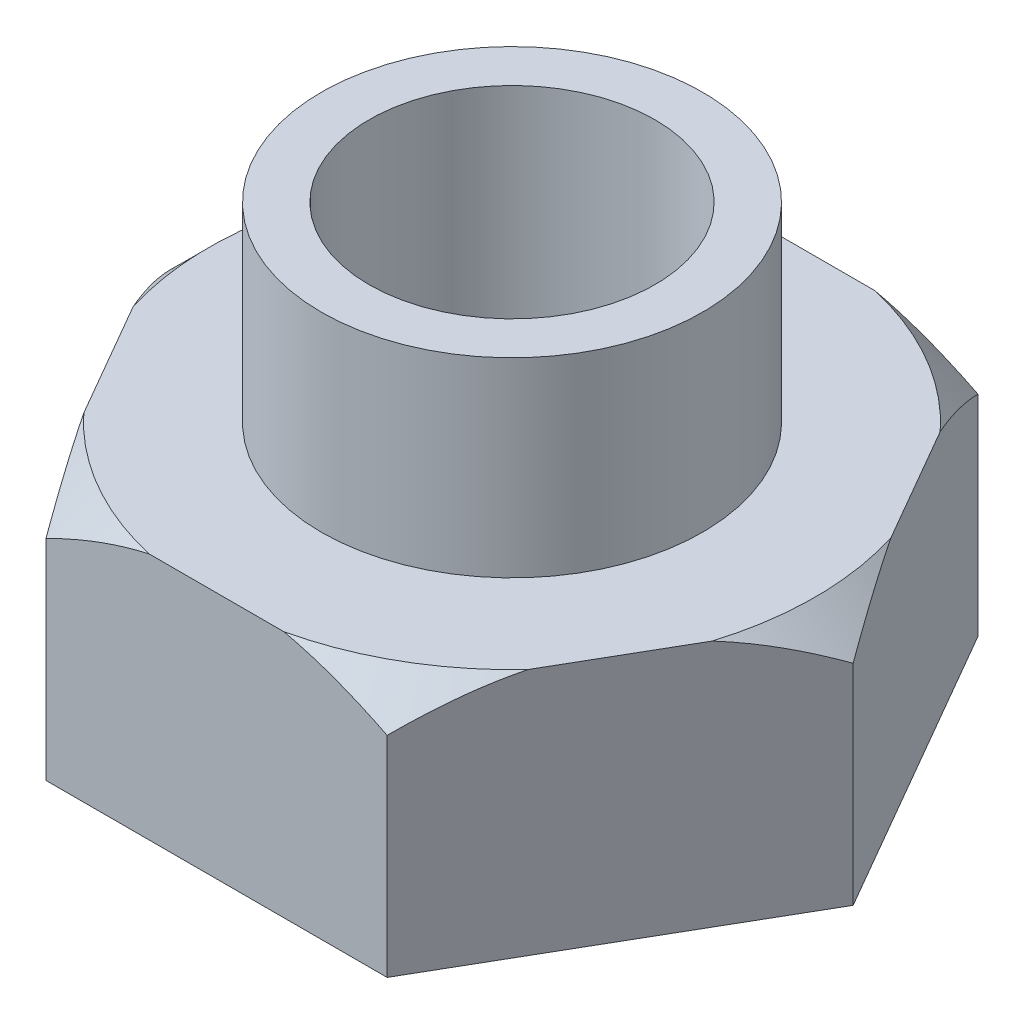
ISO-10303-21;
HEADER;
FILE_DESCRIPTION(('STEP AP214'),'2;1');
FILE_NAME('part.step','',(''),(''),'','','');
FILE_SCHEMA(('AUTOMOTIVE_DESIGN { 1 0 10303 214 1 1 1 1 }'));
ENDSEC;
DATA;
#1=APPLICATION_CONTEXT('core data for automotive mechanical design processes');
#2=APPLICATION_PROTOCOL_DEFINITION('international standard','automotive_design',2000,#1);
#3=PRODUCT_CONTEXT('',#1,'mechanical');
#4=PRODUCT('Part','Part','',(#3));
#5=PRODUCT_RELATED_PRODUCT_CATEGORY('part','',(#4));
#6=PRODUCT_DEFINITION_FORMATION('','',#4);
#7=PRODUCT_DEFINITION_CONTEXT('part definition',#1,'design');
#8=PRODUCT_DEFINITION('design','',#6,#7);
#9=PRODUCT_DEFINITION_SHAPE('','',#8);
#10=(LENGTH_UNIT() NAMED_UNIT(*) SI_UNIT(.MILLI.,.METRE.));
#11=(NAMED_UNIT(*) PLANE_ANGLE_UNIT() SI_UNIT($,.RADIAN.));
#12=(NAMED_UNIT(*) SI_UNIT($,.STERADIAN.) SOLID_ANGLE_UNIT());
#13=UNCERTAINTY_MEASURE_WITH_UNIT(LENGTH_MEASURE(1.E-05),#10,'distance_accuracy_value','');
#14=(GEOMETRIC_REPRESENTATION_CONTEXT(3) GLOBAL_UNCERTAINTY_ASSIGNED_CONTEXT((#13)) GLOBAL_UNIT_ASSIGNED_CONTEXT((#10,
#11,#12)) REPRESENTATION_CONTEXT('',''));
#15=CARTESIAN_POINT('',(0.,0.,0.));
#16=DIRECTION('',(0.,0.,1.));
#17=DIRECTION('',(1.,0.,0.));
#18=AXIS2_PLACEMENT_3D('',#15,#16,#17);
#19=CARTESIAN_POINT('',(44.7446458621968,65.,77.4999999999994));
#20=DIRECTION('',(-0.866025403784441,0.,-0.499999999999995));
#21=DIRECTION('',(-0.499999999999995,0.,0.866025403784441));
#22=AXIS2_PLACEMENT_3D('',#19,#20,#21);
#23=PLANE('',#22);
#24=DIRECTION('',(0.,-1.,0.));
#25=VECTOR('',#24,1.);
#26=CARTESIAN_POINT('',(89.4892917243919,65.,0.));
#27=LINE('',#26,#25);
#28=CARTESIAN_POINT('',(89.4892917243919,55.,0.));
#29=VERTEX_POINT('',#28);
#30=CARTESIAN_POINT('',(89.4892917243919,0.,0.));
#31=VERTEX_POINT('',#30);
#32=EDGE_CURVE('E143',#29,#31,#27,.T.);
#33=ORIENTED_EDGE('',*,*,#32,.F.);
#34=CARTESIAN_POINT('',(89.4896958695803,54.9995958520738,-0.000699999999991474));
#35=CARTESIAN_POINT('',(89.1050569011815,55.384232517878,0.66551423583768));
#36=CARTESIAN_POINT('',(88.7189364550444,55.7629268498045,1.3342944663882));
#37=CARTESIAN_POINT('',(87.9436118096002,56.5075695846921,2.6771961446579));
#38=CARTESIAN_POINT('',(87.5544074515959,56.8735173264198,3.35131786724859));
#39=CARTESIAN_POINT('',(86.3816703612672,57.9512361118258,5.38255809161848));
#40=CARTESIAN_POINT('',(85.5933844357646,58.6425099930155,6.74790936548051));
#41=CARTESIAN_POINT('',(83.9991957948086,59.9660808701838,9.5091250884655));
#42=CARTESIAN_POINT('',(83.1932180565484,60.5980175412681,10.9051194809016));
#43=CARTESIAN_POINT('',(81.5680190304813,61.7892574339015,13.7200467664614));
#44=CARTESIAN_POINT('',(80.7487997889563,62.3485717597596,15.1389761153207));
#45=CARTESIAN_POINT('',(79.1103568714706,63.3768133122282,17.9768424937074));
#46=CARTESIAN_POINT('',(78.2913355438789,63.8470227393717,19.3954290455787));
#47=CARTESIAN_POINT('',(76.6416960682088,64.6983659711274,22.2526884316105));
#48=CARTESIAN_POINT('',(75.8110773527314,65.0794954012273,23.6913622485351));
#49=CARTESIAN_POINT('',(74.1419261281375,65.7429749630036,26.5824169750476));
#50=CARTESIAN_POINT('',(73.3034167901991,66.0255550118445,28.0347577509778));
#51=CARTESIAN_POINT('',(72.0404178857128,66.3706991110335,30.222336023452));
#52=CARTESIAN_POINT('',(71.6185471841566,66.4726259396869,30.953037512772));
#53=CARTESIAN_POINT('',(70.7734023724707,66.6495728557959,32.4168712663654));
#54=CARTESIAN_POINT('',(70.3501283084779,66.7245938191311,33.1500034507269));
#55=CARTESIAN_POINT('',(69.3198595258822,66.8735850860353,34.934481327635));
#56=CARTESIAN_POINT('',(68.7123296648378,66.9331590965551,35.986753914079));
#57=CARTESIAN_POINT('',(67.4965912091334,66.9951027274195,38.0924746880745));
#58=CARTESIAN_POINT('',(66.8883826620717,66.9974761347221,39.1459227931829));
#59=CARTESIAN_POINT('',(65.6723582214112,66.9449878171684,41.2521389076525));
#60=CARTESIAN_POINT('',(65.0645425552175,66.8901049925216,42.3049065231363));
#61=CARTESIAN_POINT('',(63.8508418661291,66.7239135417307,44.4070977818189));
#62=CARTESIAN_POINT('',(63.2449568765147,66.6126039481607,45.4565213673744));
#63=CARTESIAN_POINT('',(62.0356913717897,66.3350673133356,47.5510306613984));
#64=CARTESIAN_POINT('',(61.4323142553563,66.1687812755619,48.5961104831855));
#65=CARTESIAN_POINT('',(60.2297807669441,65.7836740867063,50.6789595829185));
#66=CARTESIAN_POINT('',(59.6306244176872,65.5648526530292,51.716728821509));
#67=CARTESIAN_POINT('',(58.4374666339414,65.0775745440043,53.783338724403));
#68=CARTESIAN_POINT('',(57.8434646138622,64.8091235865246,54.8121804029787));
#69=CARTESIAN_POINT('',(56.6612309620784,64.2258074053077,56.859869154286));
#70=CARTESIAN_POINT('',(56.0729992207842,63.9109430648839,57.8787164168322));
#71=CARTESIAN_POINT('',(54.5585629876424,63.0403145468804,60.5017969174572));
#72=CARTESIAN_POINT('',(53.6370457311653,62.4517774794746,62.097911625727));
#73=CARTESIAN_POINT('',(51.8106211510816,61.1799054118424,65.2613717946247));
#74=CARTESIAN_POINT('',(50.9057143300028,60.4965675488719,66.8287163848488));
#75=CARTESIAN_POINT('',(49.5622431172167,59.4113553178228,69.1556767839005));
#76=CARTESIAN_POINT('',(49.117397603969,59.040191225619,69.9261718143645));
#77=CARTESIAN_POINT('',(48.2317466148789,58.2789854692033,71.4601643252423));
#78=CARTESIAN_POINT('',(47.7909412053907,57.8889434956012,72.2236616907271));
#79=CARTESIAN_POINT('',(46.9135663899273,57.0916418583381,73.743319448391));
#80=CARTESIAN_POINT('',(46.4769946210092,56.6843925705084,74.4994839333075));
#81=CARTESIAN_POINT('',(45.6077389749109,55.8537715065038,76.0050788771159));
#82=CARTESIAN_POINT('',(45.1750548191597,55.4304008970922,76.754509818507));
#83=CARTESIAN_POINT('',(44.7442417170084,54.9995958520741,77.5006999999994));
#84=B_SPLINE_CURVE_WITH_KNOTS('',3,(#34,#35,#36,#37,#38,#39,#40,#41,#42,#43,#44,#45,#46,#47,#48,
#49,#50,#51,#52,#53,#54,#55,#56,#57,#58,#59,#60,#61,#62,#63,#64,#65,#66,#67,#68,#69,#70,#71,#72,
#73,#74,#75,#76,#77,#78,#79,#80,#81,#82,#83),.UNSPECIFIED.,.F.,.F.,(4,2,2,2,2,2,2,2,2,2,2,2,2,2,
2,2,2,2,2,2,2,2,2,2,4),(0.,2.58018507787733,5.16050380491332,10.3236300809077,15.5163172070987,
20.7082094088618,25.818518425128,30.9290783441169,36.0276342118267,38.5768951357473,
41.1260730648216,44.7742371561345,48.4221597205939,52.0714270749171,55.7207569973254,
59.3740158824142,63.0272944193245,66.6801523202937,70.3329407111139,76.1339570006489,
81.9351485043351,84.8269963886027,87.7188916835263,90.6090674094769,93.4990343581846),.UNSPECIFIED.);
#85=CARTESIAN_POINT('',(75.9529392952477,65.0000000000001,23.4456501564339));
#86=VERTEX_POINT('',#85);
#87=EDGE_CURVE('E130',#29,#86,#84,.T.);
#88=ORIENTED_EDGE('',*,*,#87,.T.);
#89=DIRECTION('',(0.499999999999995,0.,-0.866025403784441));
#90=VECTOR('',#89,1.);
#91=CARTESIAN_POINT('',(44.7446458621968,65.,77.4999999999994));
#92=LINE('',#91,#90);
#93=CARTESIAN_POINT('',(58.2809982913393,65.,54.0543498435659));
#94=VERTEX_POINT('',#93);
#95=EDGE_CURVE('E169',#94,#86,#92,.T.);
#96=ORIENTED_EDGE('',*,*,#95,.F.);
#97=CARTESIAN_POINT('',(44.7446458621962,55.0000000000006,77.4999999999994));
#98=VERTEX_POINT('',#97);
#99=EDGE_CURVE('E136',#94,#98,#84,.T.);
#100=ORIENTED_EDGE('',*,*,#99,.T.);
#101=DIRECTION('',(0.,-1.,0.));
#102=VECTOR('',#101,1.);
#103=CARTESIAN_POINT('',(44.7446458621968,65.,77.4999999999994));
#104=LINE('',#103,#102);
#105=CARTESIAN_POINT('',(44.7446458621968,0.,77.4999999999994));
#106=VERTEX_POINT('',#105);
#107=EDGE_CURVE('E161',#98,#106,#104,.T.);
#108=ORIENTED_EDGE('',*,*,#107,.T.);
#109=DIRECTION('',(0.499999999999995,0.,-0.866025403784441));
#110=VECTOR('',#109,1.);
#111=CARTESIAN_POINT('',(44.7446458621968,0.,77.4999999999994));
#112=LINE('',#111,#110);
#113=EDGE_CURVE('E139',#106,#31,#112,.T.);
#114=ORIENTED_EDGE('',*,*,#113,.T.);
#115=EDGE_LOOP('',(#33,#88,#96,#100,#108,#114));
#116=FACE_BOUND('',#115,.T.);
#117=ADVANCED_FACE('F39',(#116),#23,.F.);
#118=CARTESIAN_POINT('',(89.4892917243919,65.,0.));
#119=DIRECTION('',(-0.866025403784438,0.,0.500000000000001));
#120=DIRECTION('',(0.500000000000001,0.,0.866025403784438));
#121=AXIS2_PLACEMENT_3D('',#118,#119,#120);
#122=PLANE('',#121);
#123=DIRECTION('',(0.,-1.,0.));
#124=VECTOR('',#123,1.);
#125=CARTESIAN_POINT('',(44.7446458621958,65.,-77.5));
#126=LINE('',#125,#124);
#127=CARTESIAN_POINT('',(44.7446458621951,55.0000000000006,-77.5000000000001));
#128=VERTEX_POINT('',#127);
#129=CARTESIAN_POINT('',(44.7446458621958,0.,-77.5));
#130=VERTEX_POINT('',#129);
#131=EDGE_CURVE('E151',#128,#130,#126,.T.);
#132=ORIENTED_EDGE('',*,*,#131,.F.);
#133=CARTESIAN_POINT('',(44.7442417170073,54.9995958520741,-77.5007));
#134=CARTESIAN_POINT('',(45.1288806854062,55.3842325178782,-76.8344857641623));
#135=CARTESIAN_POINT('',(45.5150011315432,55.7629268498048,-76.1657055336118));
#136=CARTESIAN_POINT('',(46.2903257769875,56.5075695846923,-74.822803855342));
#137=CARTESIAN_POINT('',(46.6795301349918,56.8735173264201,-74.1486821327513));
#138=CARTESIAN_POINT('',(47.8522672253206,57.951236111826,-72.1174419083814));
#139=CARTESIAN_POINT('',(48.6405531508232,58.6425099930157,-70.7520906345193));
#140=CARTESIAN_POINT('',(50.2347417917793,59.9660808701842,-67.9908749115343));
#141=CARTESIAN_POINT('',(51.0407195300395,60.5980175412684,-66.5948805190981));
#142=CARTESIAN_POINT('',(52.6659185561067,61.7892574339019,-63.7799532335383));
#143=CARTESIAN_POINT('',(53.4851377976317,62.34857175976,-62.3610238846789));
#144=CARTESIAN_POINT('',(55.1235807151175,63.3768133122285,-59.5231575062922));
#145=CARTESIAN_POINT('',(55.9426020427092,63.8470227393721,-58.1045709544209));
#146=CARTESIAN_POINT('',(57.5922415183793,64.6983659711277,-55.2473115683889));
#147=CARTESIAN_POINT('',(58.4228602338568,65.0794954012278,-53.8086377514643));
#148=CARTESIAN_POINT('',(60.0920114584508,65.7429749630041,-50.9175830249518));
#149=CARTESIAN_POINT('',(60.9305207963892,66.0255550118449,-49.4652422490215));
#150=CARTESIAN_POINT('',(62.1935197008756,66.3706991110339,-47.2776639765473));
#151=CARTESIAN_POINT('',(62.6153904024317,66.4726259396873,-46.5469624872273));
#152=CARTESIAN_POINT('',(63.4605352141178,66.6495728557963,-45.0831287336339));
#153=CARTESIAN_POINT('',(63.8838092781105,66.7245938191315,-44.3499965492723));
#154=CARTESIAN_POINT('',(64.9140780607063,66.8735850860356,-42.5655186723642));
#155=CARTESIAN_POINT('',(65.5216079217506,66.9331590965555,-41.5132460859202));
#156=CARTESIAN_POINT('',(66.7373463774551,66.9951027274199,-39.4075253119247));
#157=CARTESIAN_POINT('',(67.3455549245168,66.9974761347224,-38.3540772068163));
#158=CARTESIAN_POINT('',(68.5615793651773,66.9449878171687,-36.2478610923468));
#159=CARTESIAN_POINT('',(69.169395031371,66.8901049925219,-35.1950934768629));
#160=CARTESIAN_POINT('',(70.3830957204594,66.723913541731,-33.0929022181804));
#161=CARTESIAN_POINT('',(70.9889807100738,66.6126039481609,-32.0434786326249));
#162=CARTESIAN_POINT('',(72.1982462147988,66.3350673133358,-29.9489693386009));
#163=CARTESIAN_POINT('',(72.8016233312322,66.1687812755621,-28.9038895168138));
#164=CARTESIAN_POINT('',(74.0041568196444,65.7836740867065,-26.8210404170808));
#165=CARTESIAN_POINT('',(74.6033131689013,65.5648526530294,-25.7832711784903));
#166=CARTESIAN_POINT('',(75.7964709526471,65.0775745440045,-23.7166612755963));
#167=CARTESIAN_POINT('',(76.3904729727263,64.8091235865247,-22.6878195970207));
#168=CARTESIAN_POINT('',(77.5727066245101,64.2258074053079,-20.6401308457134));
#169=CARTESIAN_POINT('',(78.1609383658043,63.910943064884,-19.6212835831671));
#170=CARTESIAN_POINT('',(79.6753745989462,63.0403145468805,-16.9982030825422));
#171=CARTESIAN_POINT('',(80.5968918554233,62.4517774794747,-15.4020883742723));
#172=CARTESIAN_POINT('',(82.4233164355071,61.1799054118424,-12.2386282053747));
#173=CARTESIAN_POINT('',(83.3282232565858,60.4965675488719,-10.6712836151506));
#174=CARTESIAN_POINT('',(84.671694469372,59.4113553178227,-8.34432321609883));
#175=CARTESIAN_POINT('',(85.1165399826196,59.0401912256189,-7.57382818563485));
#176=CARTESIAN_POINT('',(86.0021909717098,58.2789854692032,-6.03983567475706));
#177=CARTESIAN_POINT('',(86.442996381198,57.8889434956011,-5.2763383092723));
#178=CARTESIAN_POINT('',(87.3203711966614,57.091641858338,-3.75668055160835));
#179=CARTESIAN_POINT('',(87.7569429655795,56.6843925705082,-3.00051606669191));
#180=CARTESIAN_POINT('',(88.6261986116778,55.8537715065036,-1.49492112288352));
#181=CARTESIAN_POINT('',(89.058882767429,55.430400897092,-0.745490181492405));
#182=CARTESIAN_POINT('',(89.4896958695803,54.9995958520738,0.000699999999990359));
#183=B_SPLINE_CURVE_WITH_KNOTS('',3,(#133,#134,#135,#136,#137,#138,#139,#140,#141,#142,#143,
#144,#145,#146,#147,#148,#149,#150,#151,#152,#153,#154,#155,#156,#157,#158,#159,#160,#161,#162,
#163,#164,#165,#166,#167,#168,#169,#170,#171,#172,#173,#174,#175,#176,#177,#178,#179,#180,#181,
#182),.UNSPECIFIED.,.F.,.F.,(4,2,2,2,2,2,2,2,2,2,2,2,2,2,2,2,2,2,2,2,2,2,2,2,4),(0.,
2.5801850778774,5.16050380491346,10.323630080908,15.5163172070991,20.7082094088623,
25.8185184251287,30.9290783441177,36.0276342118276,38.5768951357483,41.1260730648227,
44.7742371561356,48.422159720595,52.0714270749182,55.7207569973265,59.3740158824153,
63.0272944193256,66.6801523202947,70.3329407111149,76.1339570006501,81.9351485043363,
84.8269963886039,87.7188916835275,90.6090674094781,93.4990343581859),.UNSPECIFIED.);
#184=CARTESIAN_POINT('',(58.2809982913408,65.0000000000003,-54.0543498435619));
#185=VERTEX_POINT('',#184);
#186=EDGE_CURVE('E148',#128,#185,#183,.T.);
#187=ORIENTED_EDGE('',*,*,#186,.T.);
#188=DIRECTION('',(-0.500000000000001,0.,-0.866025403784438));
#189=VECTOR('',#188,1.);
#190=CARTESIAN_POINT('',(89.4892917243919,65.,0.));
#191=LINE('',#190,#189);
#192=CARTESIAN_POINT('',(75.9529392952479,65.,-23.4456501564357));
#193=VERTEX_POINT('',#192);
#194=EDGE_CURVE('E146',#193,#185,#191,.T.);
#195=ORIENTED_EDGE('',*,*,#194,.F.);
#196=EDGE_CURVE('E128',#193,#29,#183,.T.);
#197=ORIENTED_EDGE('',*,*,#196,.T.);
#198=ORIENTED_EDGE('',*,*,#32,.T.);
#199=DIRECTION('',(-0.500000000000001,0.,-0.866025403784438));
#200=VECTOR('',#199,1.);
#201=CARTESIAN_POINT('',(89.4892917243919,0.,0.));
#202=LINE('',#201,#200);
#203=EDGE_CURVE('E177',#31,#130,#202,.T.);
#204=ORIENTED_EDGE('',*,*,#203,.T.);
#205=EDGE_LOOP('',(#132,#187,#195,#197,#198,#204));
#206=FACE_BOUND('',#205,.T.);
#207=ADVANCED_FACE('F141',(#206),#122,.F.);
#208=CARTESIAN_POINT('',(44.7446458621958,65.,-77.5));
#209=DIRECTION('',(0.,0.,1.));
#210=DIRECTION('',(1.,0.,0.));
#211=AXIS2_PLACEMENT_3D('',#208,#209,#210);
#212=PLANE('',#211);
#213=DIRECTION('',(0.,-1.,0.));
#214=VECTOR('',#213,1.);
#215=CARTESIAN_POINT('',(-44.7446458621963,65.,-77.4999999999997));
#216=LINE('',#215,#214);
#217=CARTESIAN_POINT('',(-44.7446458621964,55.0000000000017,-77.4999999999985));
#218=VERTEX_POINT('',#217);
#219=CARTESIAN_POINT('',(-44.7446458621963,0.,-77.4999999999997));
#220=VERTEX_POINT('',#219);
#221=EDGE_CURVE('E153',#218,#220,#216,.T.);
#222=ORIENTED_EDGE('',*,*,#221,.F.);
#223=CARTESIAN_POINT('',(-44.7453458621963,54.9996499979474,-77.4999999999997));
#224=CARTESIAN_POINT('',(-43.9760695572355,55.3842851497342,-77.4999999999997));
#225=CARTESIAN_POINT('',(-43.2038303071979,55.7629779776519,-77.4999999999997));
#226=CARTESIAN_POINT('',(-41.6531843239878,56.5076177284011,-77.4999999999997));
#227=CARTESIAN_POINT('',(-40.8747772734231,56.8735639900025,-77.4999999999997));
#228=CARTESIAN_POINT('',(-38.5293081320624,57.9512783740178,-77.4999999999997));
#229=CARTESIAN_POINT('',(-36.9527396928439,58.6425493761392,-77.4999999999997));
#230=CARTESIAN_POINT('',(-33.7643694377149,59.9661146065135,-77.4999999999997));
#231=CARTESIAN_POINT('',(-32.1524175779432,60.5980485133328,-77.4999999999997));
#232=CARTESIAN_POINT('',(-28.9020268964806,61.7892830946886,-77.4999999999997));
#233=CARTESIAN_POINT('',(-27.2635921673161,62.3485948734572,-77.4999999999997));
#234=CARTESIAN_POINT('',(-23.9867137819192,63.3768316998033,-77.4999999999998));
#235=CARTESIAN_POINT('',(-22.3486748177866,63.8470389362197,-77.4999999999998));
#236=CARTESIAN_POINT('',(-19.0494033928837,64.6983781174482,-77.4999999999998));
#237=CARTESIAN_POINT('',(-17.388169797329,65.0795056877904,-77.4999999999998));
#238=CARTESIAN_POINT('',(-14.049875116774,65.7429819452449,-77.4999999999998));
#239=CARTESIAN_POINT('',(-12.3728603734853,66.0255605469421,-77.4999999999998));
#240=CARTESIAN_POINT('',(-9.84686854040535,66.3707028270972,-77.4999999999998));
#241=CARTESIAN_POINT('',(-9.00312914174588,66.4726291080458,-77.4999999999998));
#242=CARTESIAN_POINT('',(-7.31284354886708,66.649575052545,-77.4999999999998));
#243=CARTESIAN_POINT('',(-6.46629744692031,66.7245955919619,-77.4999999999998));
#244=CARTESIAN_POINT('',(-4.40576205819575,66.8735861857652,-77.4999999999998));
#245=CARTESIAN_POINT('',(-3.1907024854887,66.9331598864815,-77.4999999999998));
#246=CARTESIAN_POINT('',(-0.759225886909656,66.9951029107093,-77.4999999999998));
#247=CARTESIAN_POINT('',(0.457191043767058,66.9974760211513,-77.4999999999999));
#248=CARTESIAN_POINT('',(2.88923958315435,66.9449871273412,-77.4999999999999));
#249=CARTESIAN_POINT('',(4.10487073705146,66.8901040233805,-77.4999999999999));
#250=CARTESIAN_POINT('',(6.53227174643624,66.7239120356365,-77.4999999999999));
#251=CARTESIAN_POINT('',(7.74404153536368,66.6126021844357,-77.4999999999999));
#252=CARTESIAN_POINT('',(10.1625721431761,66.3350650601255,-77.4999999999999));
#253=CARTESIAN_POINT('',(11.3693261647569,66.1687787910458,-77.4999999999999));
#254=CARTESIAN_POINT('',(13.7743927126454,65.7836711672154,-77.4999999999999));
#255=CARTESIAN_POINT('',(14.972705193508,65.5648495298615,-77.4999999999999));
#256=CARTESIAN_POINT('',(17.3590203213371,65.0775710420286,-77.4999999999999));
#257=CARTESIAN_POINT('',(18.5470241394877,64.8091199094287,-77.4999999999999));
#258=CARTESIAN_POINT('',(20.9114909972896,64.2258034061374,-77.4999999999999));
#259=CARTESIAN_POINT('',(22.087954256126,63.9109389187827,-77.4999999999999));
#260=CARTESIAN_POINT('',(25.1168154729186,63.0403131233306,-77.4999999999999));
#261=CARTESIAN_POINT('',(26.9598391378766,62.451779570053,-77.4999999999999));
#262=CARTESIAN_POINT('',(30.6126669880817,61.1799156064398,-77.5));
#263=CARTESIAN_POINT('',(32.422470168504,60.4965823340158,-77.5));
#264=CARTESIAN_POINT('',(35.1093971986642,59.4113776223587,-77.5));
#265=CARTESIAN_POINT('',(35.9990831452034,59.0402161401431,-77.5));
#266=CARTESIAN_POINT('',(37.7703750552121,58.2790157918041,-77.5));
#267=CARTESIAN_POINT('',(38.6519808859771,57.8889766162993,-77.5));
#268=CARTESIAN_POINT('',(40.4067206451056,57.0916807326168,-77.5));
#269=CARTESIAN_POINT('',(41.2798592991794,56.6844343999014,-77.5));
#270=CARTESIAN_POINT('',(43.0183609076701,55.8538193905504,-77.5));
#271=CARTESIAN_POINT('',(43.8837244192146,55.4304518806497,-77.5));
#272=CARTESIAN_POINT('',(44.7453458621957,54.999649997947,-77.5));
#273=B_SPLINE_CURVE_WITH_KNOTS('',3,(#223,#224,#225,#226,#227,#228,#229,#230,#231,#232,#233,
#234,#235,#236,#237,#238,#239,#240,#241,#242,#243,#244,#245,#246,#247,#248,#249,#250,#251,#252,
#253,#254,#255,#256,#257,#258,#259,#260,#261,#262,#263,#264,#265,#266,#267,#268,#269,#270,#271,
#272),.UNSPECIFIED.,.F.,.F.,(4,2,2,2,2,2,2,2,2,2,2,2,2,2,2,2,2,2,2,2,2,2,2,2,4),(0.,
2.58017866800631,5.16049098446339,10.3236044215025,15.5162784245933,20.7081575084055,
25.8184540791857,30.9290015505852,36.0275450850208,38.5767998443854,41.1259716099769,
44.7741352081296,48.4220572811538,52.0713241390379,55.7206535644845,59.3739119173562,
63.0271899226149,66.6800472909387,70.3328351472347,76.1338172863219,81.9349746003783,
84.8268054075534,87.7186836242186,90.6088423269195,93.4987922567944),.UNSPECIFIED.);
#274=CARTESIAN_POINT('',(-17.6719410039009,65.0000000000012,-77.4999999999998));
#275=VERTEX_POINT('',#274);
#276=EDGE_CURVE('E202',#218,#275,#273,.T.);
#277=ORIENTED_EDGE('',*,*,#276,.T.);
#278=DIRECTION('',(-1.,0.,0.));
#279=VECTOR('',#278,1.);
#280=CARTESIAN_POINT('',(44.7446458621958,65.,-77.5));
#281=LINE('',#280,#279);
#282=CARTESIAN_POINT('',(17.671941003902,65.,-77.4999999999999));
#283=VERTEX_POINT('',#282);
#284=EDGE_CURVE('E188',#283,#275,#281,.T.);
#285=ORIENTED_EDGE('',*,*,#284,.F.);
#286=EDGE_CURVE('E198',#283,#128,#273,.T.);
#287=ORIENTED_EDGE('',*,*,#286,.T.);
#288=ORIENTED_EDGE('',*,*,#131,.T.);
#289=DIRECTION('',(-1.,0.,0.));
#290=VECTOR('',#289,1.);
#291=CARTESIAN_POINT('',(44.7446458621958,0.,-77.5));
#292=LINE('',#291,#290);
#293=EDGE_CURVE('E176',#130,#220,#292,.T.);
#294=ORIENTED_EDGE('',*,*,#293,.T.);
#295=EDGE_LOOP('',(#222,#277,#285,#287,#288,#294));
#296=FACE_BOUND('',#295,.T.);
#297=ADVANCED_FACE('F253',(#296),#212,.F.);
#298=CARTESIAN_POINT('',(-44.7446458621963,65.,-77.4999999999997));
#299=DIRECTION('',(0.866025403784442,0.,0.499999999999995));
#300=DIRECTION('',(0.499999999999995,0.,-0.866025403784442));
#301=AXIS2_PLACEMENT_3D('',#298,#299,#300);
#302=PLANE('',#301);
#303=DIRECTION('',(0.,-1.,0.));
#304=VECTOR('',#303,1.);
#305=CARTESIAN_POINT('',(-89.4892917243919,65.,6.24900384164007E-13));
#306=LINE('',#305,#304);
#307=CARTESIAN_POINT('',(-89.4892917243905,55.0000000000022,1.85268467234323E-12));
#308=VERTEX_POINT('',#307);
#309=CARTESIAN_POINT('',(-89.4892917243919,0.,6.24900384164007E-13));
#310=VERTEX_POINT('',#309);
#311=EDGE_CURVE('E156',#308,#310,#306,.T.);
#312=ORIENTED_EDGE('',*,*,#311,.F.);
#313=CARTESIAN_POINT('',(-89.4896958695803,54.9995958520747,0.0007000000006249));
#314=CARTESIAN_POINT('',(-89.1050569011815,55.3842325178789,-0.66551423583707));
#315=CARTESIAN_POINT('',(-88.7189364550444,55.7629268498054,-1.33429446638762));
#316=CARTESIAN_POINT('',(-87.9436118096002,56.507569584693,-2.67719614465738));
#317=CARTESIAN_POINT('',(-87.5544074515959,56.8735173264207,-3.35131786724809));
#318=CARTESIAN_POINT('',(-86.3816703612671,57.9512361118266,-5.38255809161807));
#319=CARTESIAN_POINT('',(-85.5933844357644,58.6425099930163,-6.74790936548013));
#320=CARTESIAN_POINT('',(-83.9991957948084,59.9660808701847,-9.50912508846523));
#321=CARTESIAN_POINT('',(-83.1932180565481,60.5980175412689,-10.9051194809014));
#322=CARTESIAN_POINT('',(-81.568019030481,61.7892574339023,-13.7200467664613));
#323=CARTESIAN_POINT('',(-80.7487997889559,62.3485717597605,-15.1389761153207));
#324=CARTESIAN_POINT('',(-79.1103568714702,63.376813312229,-17.9768424937074));
#325=CARTESIAN_POINT('',(-78.2913355438785,63.8470227393725,-19.3954290455788));
#326=CARTESIAN_POINT('',(-76.6416960682083,64.6983659711281,-22.2526884316108));
#327=CARTESIAN_POINT('',(-75.8110773527308,65.0794954012281,-23.6913622485354));
#328=CARTESIAN_POINT('',(-74.1419261281369,65.7429749630044,-26.582416975048));
#329=CARTESIAN_POINT('',(-73.3034167901985,66.0255550118452,-28.0347577509782));
#330=CARTESIAN_POINT('',(-72.0404178857121,66.3706991110342,-30.2223360234525));
#331=CARTESIAN_POINT('',(-71.618547184156,66.4726259396876,-30.9530375127725));
#332=CARTESIAN_POINT('',(-70.7734023724699,66.6495728557966,-32.416871266366));
#333=CARTESIAN_POINT('',(-70.3501283084772,66.7245938191318,-33.1500034507276));
#334=CARTESIAN_POINT('',(-69.3198595258814,66.8735850860359,-34.9344813276357));
#335=CARTESIAN_POINT('',(-68.712329664837,66.9331590965557,-35.9867539140797));
#336=CARTESIAN_POINT('',(-67.4965912091325,66.9951027274201,-38.0924746880753));
#337=CARTESIAN_POINT('',(-66.8883826620708,66.9974761347226,-39.1459227931838));
#338=CARTESIAN_POINT('',(-65.6723582214103,66.9449878171689,-41.2521389076534));
#339=CARTESIAN_POINT('',(-65.0645425552166,66.8901049925221,-42.3049065231373));
#340=CARTESIAN_POINT('',(-63.8508418661281,66.7239135417311,-44.4070977818199));
#341=CARTESIAN_POINT('',(-63.2449568765137,66.6126039481611,-45.4565213673755));
#342=CARTESIAN_POINT('',(-62.0356913717887,66.3350673133359,-47.5510306613995));
#343=CARTESIAN_POINT('',(-61.4323142553553,66.1687812755622,-48.5961104831866));
#344=CARTESIAN_POINT('',(-60.229780766943,65.7836740867065,-50.6789595829198));
#345=CARTESIAN_POINT('',(-59.6306244176861,65.5648526530294,-51.7167288215103));
#346=CARTESIAN_POINT('',(-58.4374666339402,65.0775745440045,-53.7833387244044));
#347=CARTESIAN_POINT('',(-57.8434646138611,64.8091235865247,-54.8121804029801));
#348=CARTESIAN_POINT('',(-56.6612309620772,64.2258074053078,-56.8598691542875));
#349=CARTESIAN_POINT('',(-56.072999220783,63.9109430648839,-57.8787164168338));
#350=CARTESIAN_POINT('',(-54.5585629876412,63.0403145468804,-60.5017969174586));
#351=CARTESIAN_POINT('',(-53.6370457311641,62.4517774794747,-62.0979116257284));
#352=CARTESIAN_POINT('',(-51.8106211510805,61.1799054118425,-65.2613717946258));
#353=CARTESIAN_POINT('',(-50.9057143300018,60.496567548872,-66.8287163848498));
#354=CARTESIAN_POINT('',(-49.5622431172158,59.4113553178229,-69.1556767839014));
#355=CARTESIAN_POINT('',(-49.1173976039682,59.0401912256192,-69.9261718143653));
#356=CARTESIAN_POINT('',(-48.2317466148781,58.2789854692035,-71.460164325243));
#357=CARTESIAN_POINT('',(-47.7909412053899,57.8889434956014,-72.2236616907278));
#358=CARTESIAN_POINT('',(-46.9135663899266,57.0916418583384,-73.7433194483916));
#359=CARTESIAN_POINT('',(-46.4769946210085,56.6843925705087,-74.499483933308));
#360=CARTESIAN_POINT('',(-45.6077389749103,55.8537715065042,-76.0050788771163));
#361=CARTESIAN_POINT('',(-45.1750548191591,55.4304008970926,-76.7545098185074));
#362=CARTESIAN_POINT('',(-44.7442417170079,54.9995958520745,-77.5006999999997));
#363=B_SPLINE_CURVE_WITH_KNOTS('',3,(#313,#314,#315,#316,#317,#318,#319,#320,#321,#322,#323,
#324,#325,#326,#327,#328,#329,#330,#331,#332,#333,#334,#335,#336,#337,#338,#339,#340,#341,#342,
#343,#344,#345,#346,#347,#348,#349,#350,#351,#352,#353,#354,#355,#356,#357,#358,#359,#360,#361,
#362),.UNSPECIFIED.,.F.,.F.,(4,2,2,2,2,2,2,2,2,2,2,2,2,2,2,2,2,2,2,2,2,2,2,2,4),(0.,
2.58018507787741,5.16050380491349,10.323630080908,15.5163172070992,20.7082094088625,
25.8185184251289,30.9290783441179,36.0276342118279,38.5768951357486,41.126073064823,
44.7742371561361,48.4221597205955,52.0714270749189,55.7207569973273,59.3740158824162,
63.0272944193267,66.680152320296,70.3329407111163,76.1339570006511,81.9351485043369,
84.8269963886043,87.7188916835276,90.6090674094781,93.4990343581856),.UNSPECIFIED.);
#364=CARTESIAN_POINT('',(-75.9529392952439,65.0000000000019,-23.4456501564411));
#365=VERTEX_POINT('',#364);
#366=EDGE_CURVE('E243',#308,#365,#363,.T.);
#367=ORIENTED_EDGE('',*,*,#366,.T.);
#368=DIRECTION('',(-0.499999999999995,0.,0.866025403784442));
#369=VECTOR('',#368,1.);
#370=CARTESIAN_POINT('',(-44.7446458621963,65.,-77.4999999999997));
#371=LINE('',#370,#369);
#372=CARTESIAN_POINT('',(-58.2809982913441,65.,-54.054349843557));
#373=VERTEX_POINT('',#372);
#374=EDGE_CURVE('E190',#373,#365,#371,.T.);
#375=ORIENTED_EDGE('',*,*,#374,.F.);
#376=EDGE_CURVE('E249',#373,#218,#363,.T.);
#377=ORIENTED_EDGE('',*,*,#376,.T.);
#378=ORIENTED_EDGE('',*,*,#221,.T.);
#379=DIRECTION('',(-0.499999999999995,0.,0.866025403784442));
#380=VECTOR('',#379,1.);
#381=CARTESIAN_POINT('',(-44.7446458621963,0.,-77.4999999999997));
#382=LINE('',#381,#380);
#383=EDGE_CURVE('E173',#220,#310,#382,.T.);
#384=ORIENTED_EDGE('',*,*,#383,.T.);
#385=EDGE_LOOP('',(#312,#367,#375,#377,#378,#384));
#386=FACE_BOUND('',#385,.T.);
#387=ADVANCED_FACE('F252',(#386),#302,.F.);
#388=CARTESIAN_POINT('',(-89.4892917243919,65.,6.24900384164007E-13));
#389=DIRECTION('',(0.866025403784434,0.,-0.500000000000007));
#390=DIRECTION('',(-0.500000000000007,0.,-0.866025403784435));
#391=AXIS2_PLACEMENT_3D('',#388,#389,#390);
#392=PLANE('',#391);
#393=DIRECTION('',(0.,-1.,0.));
#394=VECTOR('',#393,1.);
#395=CARTESIAN_POINT('',(-44.7446458621952,65.,77.5000000000003));
#396=LINE('',#395,#394);
#397=CARTESIAN_POINT('',(-44.7446458621931,55.0000000000017,77.5000000000004));
#398=VERTEX_POINT('',#397);
#399=CARTESIAN_POINT('',(-44.7446458621952,0.,77.5000000000003));
#400=VERTEX_POINT('',#399);
#401=EDGE_CURVE('E163',#398,#400,#396,.T.);
#402=ORIENTED_EDGE('',*,*,#401,.F.);
#403=CARTESIAN_POINT('',(-44.7442417170068,54.9995958520745,77.5007000000003));
#404=CARTESIAN_POINT('',(-45.1288806854056,55.3842325178786,76.8344857641627));
#405=CARTESIAN_POINT('',(-45.5150011315427,55.7629268498052,76.1657055336121));
#406=CARTESIAN_POINT('',(-46.2903257769869,56.5075695846928,74.8228038553424));
#407=CARTESIAN_POINT('',(-46.6795301349913,56.8735173264205,74.1486821327517));
#408=CARTESIAN_POINT('',(-47.85226722532,57.9512361118264,72.1174419083818));
#409=CARTESIAN_POINT('',(-48.6405531508227,58.6425099930161,70.7520906345197));
#410=CARTESIAN_POINT('',(-50.2347417917788,59.9660808701845,67.9908749115347));
#411=CARTESIAN_POINT('',(-51.040719530039,60.5980175412688,66.5948805190985));
#412=CARTESIAN_POINT('',(-52.6659185561062,61.7892574339022,63.7799532335388));
#413=CARTESIAN_POINT('',(-53.4851377976312,62.3485717597603,62.3610238846794));
#414=CARTESIAN_POINT('',(-55.123580715117,63.3768133122288,59.5231575062927));
#415=CARTESIAN_POINT('',(-55.9426020427087,63.8470227393723,58.1045709544214));
#416=CARTESIAN_POINT('',(-57.5922415183788,64.698365971128,55.2473115683895));
#417=CARTESIAN_POINT('',(-58.4228602338564,65.079495401228,53.8086377514649));
#418=CARTESIAN_POINT('',(-60.0920114584503,65.7429749630043,50.9175830249524));
#419=CARTESIAN_POINT('',(-60.9305207963887,66.0255550118451,49.4652422490222));
#420=CARTESIAN_POINT('',(-62.1935197008751,66.3706991110341,47.2776639765479));
#421=CARTESIAN_POINT('',(-62.6153904024313,66.4726259396875,46.546962487228));
#422=CARTESIAN_POINT('',(-63.4605352141173,66.6495728557965,45.0831287336346));
#423=CARTESIAN_POINT('',(-63.88380927811,66.7245938191317,44.349996549273));
#424=CARTESIAN_POINT('',(-64.9140780607059,66.8735850860358,42.5655186723649));
#425=CARTESIAN_POINT('',(-65.5216079217502,66.9331590965557,41.5132460859208));
#426=CARTESIAN_POINT('',(-66.7373463774548,66.9951027274201,39.4075253119253));
#427=CARTESIAN_POINT('',(-67.3455549245165,66.9974761347226,38.3540772068168));
#428=CARTESIAN_POINT('',(-68.561579365177,66.9449878171689,36.2478610923472));
#429=CARTESIAN_POINT('',(-69.1693950313708,66.8901049925221,35.1950934768633));
#430=CARTESIAN_POINT('',(-70.3830957204593,66.7239135417312,33.0929022181807));
#431=CARTESIAN_POINT('',(-70.9889807100737,66.6126039481612,32.0434786326252));
#432=CARTESIAN_POINT('',(-72.1982462147987,66.335067313336,29.9489693386011));
#433=CARTESIAN_POINT('',(-72.8016233312322,66.1687812755623,28.903889516814));
#434=CARTESIAN_POINT('',(-74.0041568196445,65.7836740867067,26.8210404170809));
#435=CARTESIAN_POINT('',(-74.6033131689014,65.5648526530296,25.7832711784904));
#436=CARTESIAN_POINT('',(-75.7964709526473,65.0775745440047,23.7166612755963));
#437=CARTESIAN_POINT('',(-76.3904729727265,64.8091235865249,22.6878195970206));
#438=CARTESIAN_POINT('',(-77.5727066245104,64.225807405308,20.6401308457132));
#439=CARTESIAN_POINT('',(-78.1609383658046,63.9109430648842,19.621283583167));
#440=CARTESIAN_POINT('',(-79.6753745989465,63.0403145468807,16.9982030825421));
#441=CARTESIAN_POINT('',(-80.5968918554236,62.4517774794749,15.4020883742723));
#442=CARTESIAN_POINT('',(-82.4233164355072,61.1799054118427,12.2386282053748));
#443=CARTESIAN_POINT('',(-83.328223256586,60.4965675488723,10.6712836151508));
#444=CARTESIAN_POINT('',(-84.6716944693721,59.4113553178232,8.3443232160991));
#445=CARTESIAN_POINT('',(-85.1165399826197,59.0401912256194,7.57382818563516));
#446=CARTESIAN_POINT('',(-86.0021909717099,58.2789854692038,6.03983567475744));
#447=CARTESIAN_POINT('',(-86.4429963811981,57.8889434956017,5.2763383092727));
#448=CARTESIAN_POINT('',(-87.3203711966614,57.0916418583386,3.75668055160881));
#449=CARTESIAN_POINT('',(-87.7569429655795,56.6843925705089,3.0005160666924));
#450=CARTESIAN_POINT('',(-88.6261986116779,55.8537715065045,1.49492112288406));
#451=CARTESIAN_POINT('',(-89.058882767429,55.4304008970929,0.745490181492978));
#452=CARTESIAN_POINT('',(-89.4896958695803,54.9995958520747,-0.000699999999379708));
#453=B_SPLINE_CURVE_WITH_KNOTS('',3,(#403,#404,#405,#406,#407,#408,#409,#410,#411,#412,#413,
#414,#415,#416,#417,#418,#419,#420,#421,#422,#423,#424,#425,#426,#427,#428,#429,#430,#431,#432,
#433,#434,#435,#436,#437,#438,#439,#440,#441,#442,#443,#444,#445,#446,#447,#448,#449,#450,#451,
#452),.UNSPECIFIED.,.F.,.F.,(4,2,2,2,2,2,2,2,2,2,2,2,2,2,2,2,2,2,2,2,2,2,2,2,4),(0.,
2.58018507787738,5.16050380491342,10.3236300809079,15.516317207099,20.7082094088622,
25.8185184251285,30.9290783441175,36.0276342118274,38.576895135748,41.1260730648224,
44.7742371561354,48.4221597205949,52.0714270749183,55.7207569973267,59.3740158824156,
63.0272944193261,66.6801523202954,70.3329407111157,76.1339570006506,81.9351485043365,
84.826996388604,87.7188916835275,90.609067409478,93.4990343581856),.UNSPECIFIED.);
#454=CARTESIAN_POINT('',(-58.2809982913391,65.0000000000017,54.0543498435619));
#455=VERTEX_POINT('',#454);
#456=EDGE_CURVE('E235',#398,#455,#453,.T.);
#457=ORIENTED_EDGE('',*,*,#456,.T.);
#458=DIRECTION('',(0.500000000000007,0.,0.866025403784435));
#459=VECTOR('',#458,1.);
#460=CARTESIAN_POINT('',(-89.4892917243919,65.,6.24900384164007E-13));
#461=LINE('',#460,#459);
#462=CARTESIAN_POINT('',(-75.9529392952455,65.,23.4456501564401));
#463=VERTEX_POINT('',#462);
#464=EDGE_CURVE('E183',#463,#455,#461,.T.);
#465=ORIENTED_EDGE('',*,*,#464,.F.);
#466=EDGE_CURVE('E65',#463,#308,#453,.T.);
#467=ORIENTED_EDGE('',*,*,#466,.T.);
#468=ORIENTED_EDGE('',*,*,#311,.T.);
#469=DIRECTION('',(0.500000000000007,0.,0.866025403784435));
#470=VECTOR('',#469,1.);
#471=CARTESIAN_POINT('',(-89.4892917243919,0.,6.24900384164007E-13));
#472=LINE('',#471,#470);
#473=EDGE_CURVE('E167',#310,#400,#472,.T.);
#474=ORIENTED_EDGE('',*,*,#473,.T.);
#475=EDGE_LOOP('',(#402,#457,#465,#467,#468,#474));
#476=FACE_BOUND('',#475,.T.);
#477=ADVANCED_FACE('F251',(#476),#392,.F.);
#478=CARTESIAN_POINT('',(-44.7446458621952,65.,77.5000000000003));
#479=DIRECTION('',(0.,0.,-1.));
#480=DIRECTION('',(-1.,0.,0.));
#481=AXIS2_PLACEMENT_3D('',#478,#479,#480);
#482=PLANE('',#481);
#483=ORIENTED_EDGE('',*,*,#107,.F.);
#484=CARTESIAN_POINT('',(44.7453458621968,54.9996499979469,77.4999999999994));
#485=CARTESIAN_POINT('',(43.9760695572361,55.3842851497338,77.4999999999994));
#486=CARTESIAN_POINT('',(43.2038303071985,55.7629779776514,77.4999999999994));
#487=CARTESIAN_POINT('',(41.6531843239885,56.5076177284007,77.4999999999994));
#488=CARTESIAN_POINT('',(40.8747772734239,56.8735639900021,77.4999999999994));
#489=CARTESIAN_POINT('',(38.5293081320632,57.9512783740174,77.4999999999994));
#490=CARTESIAN_POINT('',(36.9527396928448,58.6425493761388,77.4999999999995));
#491=CARTESIAN_POINT('',(33.7643694377159,59.9661146065131,77.4999999999995));
#492=CARTESIAN_POINT('',(32.1524175779442,60.5980485133324,77.4999999999995));
#493=CARTESIAN_POINT('',(28.9020268964818,61.7892830946883,77.4999999999995));
#494=CARTESIAN_POINT('',(27.2635921673174,62.3485948734568,77.4999999999996));
#495=CARTESIAN_POINT('',(23.9867137819206,63.3768316998029,77.4999999999996));
#496=CARTESIAN_POINT('',(22.348674817788,63.8470389362193,77.4999999999996));
#497=CARTESIAN_POINT('',(19.0494033928852,64.6983781174479,77.4999999999996));
#498=CARTESIAN_POINT('',(17.3881697973306,65.0795056877901,77.4999999999997));
#499=CARTESIAN_POINT('',(14.0498751167757,65.7429819452447,77.4999999999997));
#500=CARTESIAN_POINT('',(12.3728603734871,66.0255605469418,77.4999999999997));
#501=CARTESIAN_POINT('',(9.8468685404072,66.370702827097,77.4999999999997));
#502=CARTESIAN_POINT('',(9.00312914174776,66.4726291080456,77.4999999999997));
#503=CARTESIAN_POINT('',(7.312843548869,66.6495750525449,77.4999999999998));
#504=CARTESIAN_POINT('',(6.46629744692226,66.7245955919618,77.4999999999998));
#505=CARTESIAN_POINT('',(4.40576205819773,66.8735861857651,77.4999999999998));
#506=CARTESIAN_POINT('',(3.19070248549068,66.9331598864814,77.4999999999998));
#507=CARTESIAN_POINT('',(0.759225886911639,66.9951029107093,77.4999999999998));
#508=CARTESIAN_POINT('',(-0.457191043765073,66.9974760211514,77.4999999999998));
#509=CARTESIAN_POINT('',(-2.88923958315236,66.9449871273412,77.4999999999999));
#510=CARTESIAN_POINT('',(-4.10487073704947,66.8901040233806,77.4999999999999));
#511=CARTESIAN_POINT('',(-6.53227174643425,66.7239120356366,77.4999999999999));
#512=CARTESIAN_POINT('',(-7.74404153536169,66.6126021844358,77.4999999999999));
#513=CARTESIAN_POINT('',(-10.1625721431741,66.3350650601257,77.5));
#514=CARTESIAN_POINT('',(-11.3693261647549,66.1687787910461,77.5));
#515=CARTESIAN_POINT('',(-13.7743927126435,65.7836711672157,77.5));
#516=CARTESIAN_POINT('',(-14.972705193506,65.5648495298618,77.5));
#517=CARTESIAN_POINT('',(-17.3590203213352,65.077571042029,77.5));
#518=CARTESIAN_POINT('',(-18.5470241394857,64.8091199094291,77.5));
#519=CARTESIAN_POINT('',(-20.9114909972876,64.2258034061379,77.5000000000001));
#520=CARTESIAN_POINT('',(-22.087954256124,63.9109389187832,77.5000000000001));
#521=CARTESIAN_POINT('',(-25.1168154729168,63.0403131233311,77.5000000000001));
#522=CARTESIAN_POINT('',(-26.9598391378749,62.4517795700535,77.5000000000001));
#523=CARTESIAN_POINT('',(-30.6126669880802,61.1799156064403,77.5000000000002));
#524=CARTESIAN_POINT('',(-32.4224701685026,60.4965823340164,77.5000000000002));
#525=CARTESIAN_POINT('',(-35.109397198663,59.4113776223592,77.5000000000002));
#526=CARTESIAN_POINT('',(-35.9990831452023,59.0402161401436,77.5000000000002));
#527=CARTESIAN_POINT('',(-37.7703750552111,58.2790157918046,77.5000000000003));
#528=CARTESIAN_POINT('',(-38.6519808859762,57.8889766162998,77.5000000000003));
#529=CARTESIAN_POINT('',(-40.4067206451047,57.0916807326173,77.5000000000003));
#530=CARTESIAN_POINT('',(-41.2798592991786,56.6844343999018,77.5000000000003));
#531=CARTESIAN_POINT('',(-43.0183609076695,55.8538193905509,77.5000000000003));
#532=CARTESIAN_POINT('',(-43.883724419214,55.4304518806501,77.5000000000003));
#533=CARTESIAN_POINT('',(-44.7453458621952,54.9996499979474,77.5000000000003));
#534=B_SPLINE_CURVE_WITH_KNOTS('',3,(#484,#485,#486,#487,#488,#489,#490,#491,#492,#493,#494,
#495,#496,#497,#498,#499,#500,#501,#502,#503,#504,#505,#506,#507,#508,#509,#510,#511,#512,#513,
#514,#515,#516,#517,#518,#519,#520,#521,#522,#523,#524,#525,#526,#527,#528,#529,#530,#531,#532,
#533),.UNSPECIFIED.,.F.,.F.,(4,2,2,2,2,2,2,2,2,2,2,2,2,2,2,2,2,2,2,2,2,2,2,2,4),(0.,
2.58017866800623,5.16049098446322,10.3236044215022,15.5162784245928,20.7081575084049,
25.8184540791849,30.9290015505842,36.0275450850196,38.5767998443842,41.1259716099756,
44.7741352081283,48.4220572811525,52.0713241390366,55.7206535644832,59.3739119173549,
63.0271899226136,66.6800472909374,70.3328351472334,76.1338172863209,81.9349746003777,
84.8268054075529,87.7186836242183,90.6088423269194,93.4987922567944),.UNSPECIFIED.);
#535=CARTESIAN_POINT('',(17.6719410039115,65.0000000000008,77.4999999999978));
#536=VERTEX_POINT('',#535);
#537=EDGE_CURVE('E408',#98,#536,#534,.T.);
#538=ORIENTED_EDGE('',*,*,#537,.T.);
#539=DIRECTION('',(1.,0.,0.));
#540=VECTOR('',#539,1.);
#541=CARTESIAN_POINT('',(-44.7446458621952,65.,77.5000000000003));
#542=LINE('',#541,#540);
#543=CARTESIAN_POINT('',(-17.6719410039086,65.,77.5));
#544=VERTEX_POINT('',#543);
#545=EDGE_CURVE('E164',#544,#536,#542,.T.);
#546=ORIENTED_EDGE('',*,*,#545,.F.);
#547=EDGE_CURVE('E53',#544,#398,#534,.T.);
#548=ORIENTED_EDGE('',*,*,#547,.T.);
#549=ORIENTED_EDGE('',*,*,#401,.T.);
#550=DIRECTION('',(1.,0.,0.));
#551=VECTOR('',#550,1.);
#552=CARTESIAN_POINT('',(-44.7446458621952,0.,77.5000000000003));
#553=LINE('',#552,#551);
#554=EDGE_CURVE('E168',#400,#106,#553,.T.);
#555=ORIENTED_EDGE('',*,*,#554,.T.);
#556=EDGE_LOOP('',(#483,#538,#546,#548,#549,#555));
#557=FACE_BOUND('',#556,.T.);
#558=ADVANCED_FACE('F291',(#557),#482,.F.);
#559=CARTESIAN_POINT('',(0.,65.,0.));
#560=DIRECTION('',(0.,1.,0.));
#561=DIRECTION('',(0.,0.,1.));
#562=AXIS2_PLACEMENT_3D('',#559,#560,#561);
#563=PLANE('',#562);
#564=CARTESIAN_POINT('',(0.,65.,0.));
#565=DIRECTION('',(0.,1.,0.));
#566=DIRECTION('',(0.,0.,1.));
#567=AXIS2_PLACEMENT_3D('',#564,#565,#566);
#568=CIRCLE('',#567,50.);
#569=CARTESIAN_POINT('',(0.,65.,50.));
#570=VERTEX_POINT('',#569);
#571=EDGE_CURVE('E402',#570,#570,#568,.T.);
#572=ORIENTED_EDGE('',*,*,#571,.F.);
#573=EDGE_LOOP('',(#572));
#574=FACE_BOUND('',#573,.T.);
#575=CARTESIAN_POINT('',(8.11850586757158E-13,65.,9.92821971190156E-13));
#576=DIRECTION('',(0.,1.,0.));
#577=DIRECTION('',(0.,0.,1.));
#578=AXIS2_PLACEMENT_3D('',#575,#576,#577);
#579=CIRCLE('',#578,79.4892917243921);
#580=EDGE_CURVE('E11',#544,#455,#579,.F.);
#581=ORIENTED_EDGE('',*,*,#580,.F.);
#582=ORIENTED_EDGE('',*,*,#545,.T.);
#583=EDGE_CURVE('E43',#94,#536,#579,.F.);
#584=ORIENTED_EDGE('',*,*,#583,.F.);
#585=ORIENTED_EDGE('',*,*,#95,.T.);
#586=EDGE_CURVE('E135',#193,#86,#579,.F.);
#587=ORIENTED_EDGE('',*,*,#586,.F.);
#588=ORIENTED_EDGE('',*,*,#194,.T.);
#589=EDGE_CURVE('E433',#283,#185,#579,.F.);
#590=ORIENTED_EDGE('',*,*,#589,.F.);
#591=ORIENTED_EDGE('',*,*,#284,.T.);
#592=EDGE_CURVE('E431',#373,#275,#579,.F.);
#593=ORIENTED_EDGE('',*,*,#592,.F.);
#594=ORIENTED_EDGE('',*,*,#374,.T.);
#595=EDGE_CURVE('E48',#463,#365,#579,.F.);
#596=ORIENTED_EDGE('',*,*,#595,.F.);
#597=ORIENTED_EDGE('',*,*,#464,.T.);
#598=EDGE_LOOP('',(#581,#582,#584,#585,#587,#588,#590,#591,#593,#594,#596,#597));
#599=FACE_BOUND('',#598,.T.);
#600=ADVANCED_FACE('F219',(#574,#599),#563,.T.);
#601=CARTESIAN_POINT('',(0.,0.,0.));
#602=DIRECTION('',(0.,1.,0.));
#603=DIRECTION('',(0.,0.,1.));
#604=AXIS2_PLACEMENT_3D('',#601,#602,#603);
#605=PLANE('',#604);
#606=CARTESIAN_POINT('',(0.,0.,0.));
#607=DIRECTION('',(0.,1.,0.));
#608=DIRECTION('',(0.,0.,1.));
#609=AXIS2_PLACEMENT_3D('',#606,#607,#608);
#610=CIRCLE('',#609,37.5);
#611=CARTESIAN_POINT('',(0.,0.,37.5));
#612=VERTEX_POINT('',#611);
#613=EDGE_CURVE('E398',#612,#612,#610,.F.);
#614=ORIENTED_EDGE('',*,*,#613,.F.);
#615=EDGE_LOOP('',(#614));
#616=FACE_BOUND('',#615,.T.);
#617=ORIENTED_EDGE('',*,*,#113,.F.);
#618=ORIENTED_EDGE('',*,*,#554,.F.);
#619=ORIENTED_EDGE('',*,*,#473,.F.);
#620=ORIENTED_EDGE('',*,*,#383,.F.);
#621=ORIENTED_EDGE('',*,*,#293,.F.);
#622=ORIENTED_EDGE('',*,*,#203,.F.);
#623=EDGE_LOOP('',(#617,#618,#619,#620,#621,#622));
#624=FACE_BOUND('',#623,.T.);
#625=ADVANCED_FACE('F311',(#616,#624),#605,.F.);
#626=CARTESIAN_POINT('',(8.11850586757158E-13,65.000000000001,0.));
#627=DIRECTION('',(0.,-1.,0.));
#628=DIRECTION('',(1.,0.,0.));
#629=AXIS2_PLACEMENT_3D('',#626,#627,#628);
#630=CONICAL_SURFACE('',#629,79.4892917243911,0.785398163397461);
#631=ORIENTED_EDGE('',*,*,#583,.T.);
#632=ORIENTED_EDGE('',*,*,#537,.F.);
#633=ORIENTED_EDGE('',*,*,#99,.F.);
#634=EDGE_LOOP('',(#631,#632,#633));
#635=FACE_BOUND('',#634,.T.);
#636=ADVANCED_FACE('F211',(#635),#630,.T.);
#637=ORIENTED_EDGE('',*,*,#196,.F.);
#638=ORIENTED_EDGE('',*,*,#586,.T.);
#639=ORIENTED_EDGE('',*,*,#87,.F.);
#640=EDGE_LOOP('',(#637,#638,#639));
#641=FACE_BOUND('',#640,.T.);
#642=ADVANCED_FACE('F126',(#641),#630,.T.);
#643=ORIENTED_EDGE('',*,*,#286,.F.);
#644=ORIENTED_EDGE('',*,*,#589,.T.);
#645=ORIENTED_EDGE('',*,*,#186,.F.);
#646=EDGE_LOOP('',(#643,#644,#645));
#647=FACE_BOUND('',#646,.T.);
#648=ADVANCED_FACE('F214',(#647),#630,.T.);
#649=ORIENTED_EDGE('',*,*,#376,.F.);
#650=ORIENTED_EDGE('',*,*,#592,.T.);
#651=ORIENTED_EDGE('',*,*,#276,.F.);
#652=EDGE_LOOP('',(#649,#650,#651));
#653=FACE_BOUND('',#652,.T.);
#654=ADVANCED_FACE('F343',(#653),#630,.T.);
#655=ORIENTED_EDGE('',*,*,#466,.F.);
#656=ORIENTED_EDGE('',*,*,#595,.T.);
#657=ORIENTED_EDGE('',*,*,#366,.F.);
#658=EDGE_LOOP('',(#655,#656,#657));
#659=FACE_BOUND('',#658,.T.);
#660=ADVANCED_FACE('F332',(#659),#630,.T.);
#661=ORIENTED_EDGE('',*,*,#547,.F.);
#662=ORIENTED_EDGE('',*,*,#580,.T.);
#663=ORIENTED_EDGE('',*,*,#456,.F.);
#664=EDGE_LOOP('',(#661,#662,#663));
#665=FACE_BOUND('',#664,.T.);
#666=ADVANCED_FACE('F213',(#665),#630,.T.);
#667=CARTESIAN_POINT('',(0.,115.,0.));
#668=DIRECTION('',(0.,-1.,0.));
#669=DIRECTION('',(0.,0.,-1.));
#670=AXIS2_PLACEMENT_3D('',#667,#668,#669);
#671=CYLINDRICAL_SURFACE('',#670,50.);
#672=CARTESIAN_POINT('',(0.,115.,0.));
#673=DIRECTION('',(0.,1.,0.));
#674=DIRECTION('',(0.,0.,1.));
#675=AXIS2_PLACEMENT_3D('',#672,#673,#674);
#676=CIRCLE('',#675,50.);
#677=CARTESIAN_POINT('',(0.,115.,50.));
#678=VERTEX_POINT('',#677);
#679=EDGE_CURVE('E404',#678,#678,#676,.T.);
#680=ORIENTED_EDGE('',*,*,#679,.F.);
#681=EDGE_LOOP('',(#680));
#682=FACE_BOUND('',#681,.T.);
#683=ORIENTED_EDGE('',*,*,#571,.T.);
#684=EDGE_LOOP('',(#683));
#685=FACE_BOUND('',#684,.T.);
#686=ADVANCED_FACE('F217',(#682,#685),#671,.T.);
#687=CARTESIAN_POINT('',(0.,115.,0.));
#688=DIRECTION('',(0.,1.,0.));
#689=DIRECTION('',(0.,0.,1.));
#690=AXIS2_PLACEMENT_3D('',#687,#688,#689);
#691=PLANE('',#690);
#692=CARTESIAN_POINT('',(0.,115.,0.));
#693=DIRECTION('',(0.,1.,0.));
#694=DIRECTION('',(0.,0.,1.));
#695=AXIS2_PLACEMENT_3D('',#692,#693,#694);
#696=CIRCLE('',#695,37.5);
#697=CARTESIAN_POINT('',(0.,115.,37.5));
#698=VERTEX_POINT('',#697);
#699=EDGE_CURVE('E399',#698,#698,#696,.T.);
#700=ORIENTED_EDGE('',*,*,#699,.F.);
#701=EDGE_LOOP('',(#700));
#702=FACE_BOUND('',#701,.T.);
#703=ORIENTED_EDGE('',*,*,#679,.T.);
#704=EDGE_LOOP('',(#703));
#705=FACE_BOUND('',#704,.T.);
#706=ADVANCED_FACE('F372',(#702,#705),#691,.T.);
#707=CARTESIAN_POINT('',(0.,-0.001000000000001,0.));
#708=DIRECTION('',(0.,1.,0.));
#709=DIRECTION('',(0.,0.,1.));
#710=AXIS2_PLACEMENT_3D('',#707,#708,#709);
#711=CYLINDRICAL_SURFACE('',#710,37.5);
#712=ORIENTED_EDGE('',*,*,#699,.T.);
#713=EDGE_LOOP('',(#712));
#714=FACE_BOUND('',#713,.T.);
#715=ORIENTED_EDGE('',*,*,#613,.T.);
#716=EDGE_LOOP('',(#715));
#717=FACE_BOUND('',#716,.T.);
#718=ADVANCED_FACE('F385',(#714,#717),#711,.F.);
#719=CLOSED_SHELL('',(#117,#207,#297,#387,#477,#558,#600,#625,#636,#642,#648,#654,#660,#666,
#686,#706,#718));
#720=MANIFOLD_SOLID_BREP('B2',#719);
#721=ADVANCED_BREP_SHAPE_REPRESENTATION('',(#18,#720),#14);
#722=SHAPE_DEFINITION_REPRESENTATION(#9,#721);
ENDSEC;
END-ISO-10303-21;
